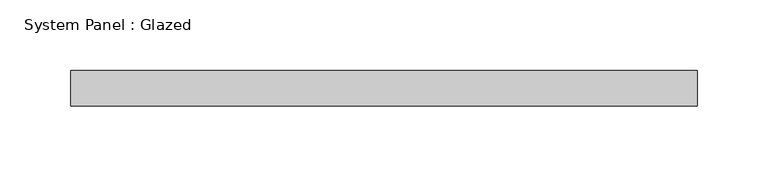
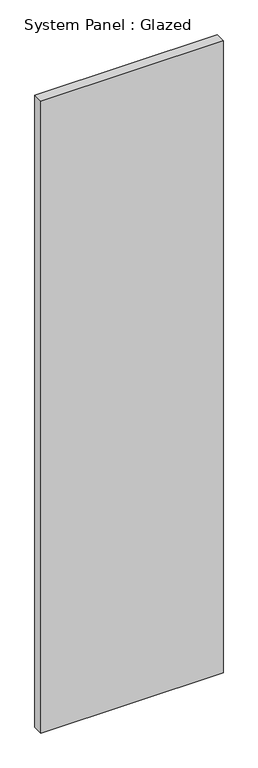
"""IFC4 building model written with IfcOpenShell, lengths in millimetres: plate geometry, System Panel : Glazed."""

from ifc_helpers import new_model, si_unit, origin, origin_with_axes, place, context, project, spatial, polyline, outline, extrude, source, transform, mapped, element, save


def system_panel_glazed_3d937ce6(model_context):
    return source(origin(), model_context, "Body", "SweptSolid", [
        extrude(outline(polyline([(222.25, 19.05), (-222.25, 19.05), (-222.25, 44.45), (222.25, 44.45), (222.25, 19.05)])), origin_with_axes(), (0.0, 0.0, 1.0), 1630.2747989),
    ])


if __name__ == "__main__":
    model = new_model("IFC4")
    model_context = context("Model", 3, world=origin())
    ifc_project = project(units=[si_unit("LENGTHUNIT", "METRE", prefix="MILLI")], contexts=[model_context])
    site = spatial("IfcSite", under=ifc_project)
    building = spatial("IfcBuilding", under=site)
    placement = place(None, origin())
    system_panel_glazed_shape = system_panel_glazed_3d937ce6(model_context)
    element("IfcPlate", 1, ObjectType="System Panel : Glazed", at=placement, inside=building, context=model_context, shape_type="MappedRepresentation", body=[
        mapped(system_panel_glazed_shape, transform((0.0, 0.0, 0.0), x_axis=(1.0, 0.0, 0.0), y_axis=(0.0, 1.0, 0.0), z_axis=(0.0, 0.0, 1.0))),
    ])
    save(model, "model.ifc")

# Revit data of these elements
# Type "System Panel : Glazed"
#   Construction Type Id = "GSP4R"
#   Analytic Construction = "1/8 in Pilkington single glazing"
#   Visual Light Transmittance = 0.9
#   Solar Heat Gain Coefficient = 0.86
#   Heat Transfer Coefficient (U) = 1.18115 BTU/(h·ft²·°F)
#   Define Thermal Properties by = 1
# Element 1 (IfcPlate, "System Panel : Glazed")
#   Materials on its faces: "Glass"
# Materials
#   "Glass": class "Glass", colour RGB 0 128 192, transparency 0.75, Description = "Soda Lime Glass", Cost = 0
